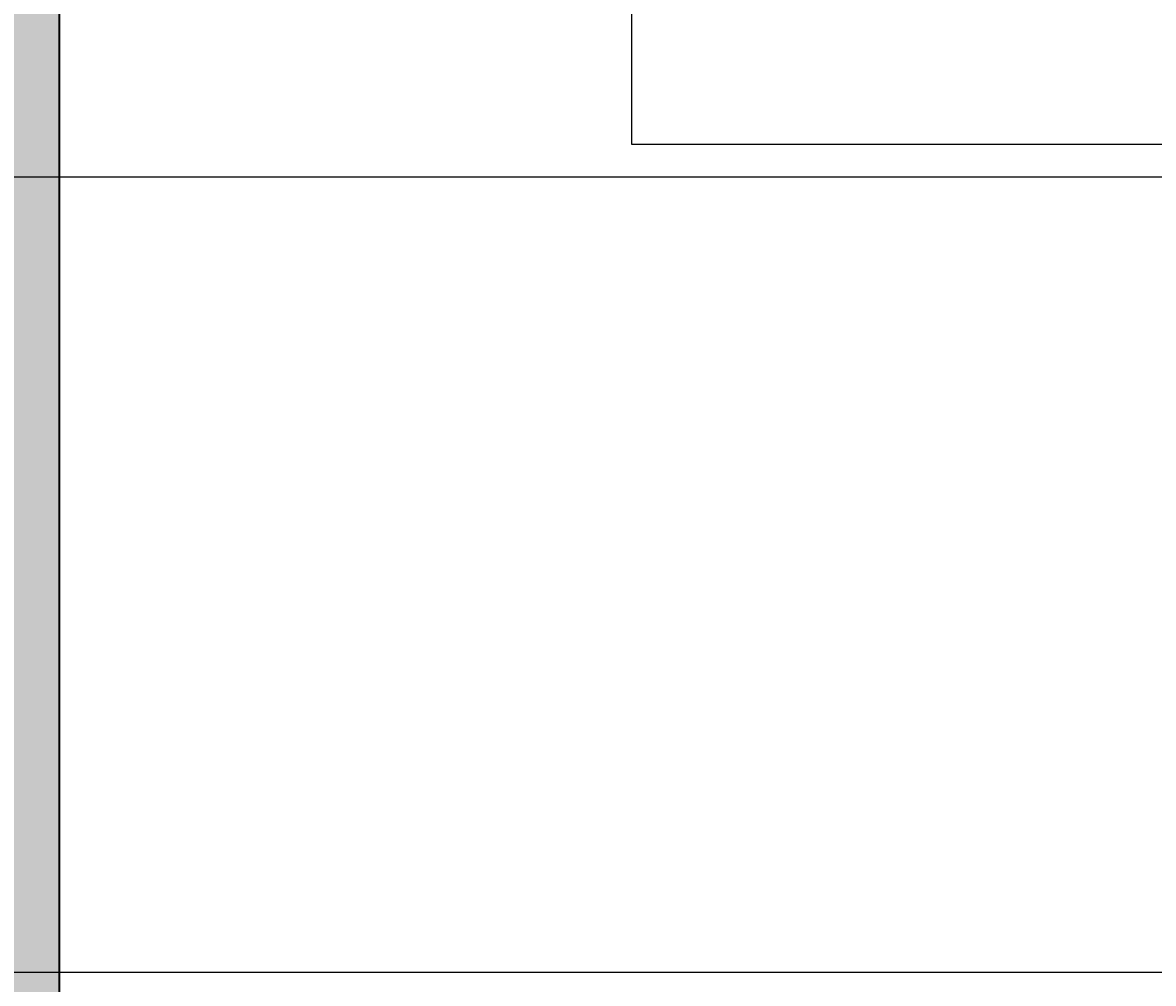
# Model space of a CAD drawing. Units: inches. Extents: x -5 to 330, y -522 to 40.
# Tile 5 of 23: x 32 to 62, y -417 to -391. Entities that reach past the tile are written whole.
import ezdxf

# ---------------------------------------------------------------- set-up
doc = ezdxf.new("R2010")
doc.units = ezdxf.units.IN
doc.header["$MEASUREMENT"] = 0
for name, color, linetype, lineweight in [('A-ANNO-DIMS', 2, 'Continuous', 18), ('A-FLOR-CASE', 8, 'Continuous', 25), ('A-WALL', 7, 'Continuous', 35)]:
    doc.layers.add(name, color=color, linetype=linetype, lineweight=lineweight)
doc.layers.add('A-WALL-PATT', color=18, linetype='Continuous', lineweight=13, true_color=0x000000)
doc.styles.get("Standard").update_dxf_attribs({"font": 'arial.ttf'})
doc.dimstyles.get("Standard").update_dxf_attribs({"dimtxt": 0.18, "dimasz": 0.18, "dimexe": 0.18, "dimexo": 0.0625, "dimgap": 0.09, "dimtad": 0, "dimtih": 1, "dimtoh": 1, "dimdec": 0, "dimzin": 0, "dimdsep": 46, "dimlunit": 3, "dimtxsty": 'Standard', "dimcen": 0.09, "dimadec": 0, "dimazin": 0, "dimtfac": 1, "dimtdec": 0, "dimtofl": 0, "dimtmove": 0, "dimatfit": 3, "dimfxl": 1, "dimtolj": 1, "dimtzin": 0, "dimarcsym": 0})

# ---------------------------------------------------------------- blocks, each defined once
blk = doc.blocks.new('*D40')
at = {"layer": 'A-ANNO-DIMS', "color": 0, "lineweight": -2, "transparency": 16777216}
for p, q in [((32.51, -246.706), (32.51, -522.309)), ((79.01, -246.706), (79.01, -522.309)), ((32.69, -522.129), (55.151, -522.129)), ((78.83, -522.129), (56.369, -522.129))]:
    blk.add_line(p, q, dxfattribs=at)
at = {"layer": 'A-ANNO-DIMS', "color": 0, "transparency": 16777216}
for points in [[(32.69, -522.099), (32.69, -522.159), (32.51, -522.129)], [(78.83, -522.099), (78.83, -522.159), (79.01, -522.129)]]:
    blk.add_solid(points, dxfattribs=at)
at = {"layer": 'Defpoints', "color": 0, "transparency": 16777216}
for p in [(32.51, -246.644), (79.01, -246.644), (79.01, -522.129)]:
    blk.add_point(p, dxfattribs=at)
at = {"layer": 'A-ANNO-DIMS', "color": 0, "transparency": 16777216, "insert": (55.76, -522.129), "char_height": 0.18, "attachment_point": 5}
blk.add_mtext('\\A1;3\'-10 1/2"', dxfattribs=at)
blk = doc.blocks.new('*D49')
at = {"layer": 'A-ANNO-DIMS', "color": 0, "lineweight": -2, "transparency": 16777216}
for p, q in [((62.948, -394.834), (-3.655, -394.834)), ((-3.475, -395.014), (-3.475, -405.506)), ((-3.475, -416.364), (-3.475, -405.872)), ((62.948, -416.544), (-3.655, -416.544))]:
    blk.add_line(p, q, dxfattribs=at)
at = {"layer": 'A-ANNO-DIMS', "color": 0, "transparency": 16777216}
for points in [[(-3.505, -395.014), (-3.445, -395.014), (-3.475, -394.834)], [(-3.505, -416.364), (-3.445, -416.364), (-3.475, -416.544)]]:
    blk.add_solid(points, dxfattribs=at)
at = {"layer": 'Defpoints', "color": 0, "transparency": 16777216}
for p in [(63.01, -394.834), (-3.475, -416.544), (63.01, -416.544)]:
    blk.add_point(p, dxfattribs=at)
at = {"layer": 'A-ANNO-DIMS', "color": 0, "transparency": 16777216, "insert": (-3.475, -405.689), "char_height": 0.18, "attachment_point": 5}
blk.add_mtext('\\A1;1\'-9 1/2"', dxfattribs=at)

msp = doc.modelspace()

# ---------------------------------------------------------------- hatches: boundary and pattern name
at = {"layer": 'A-WALL-PATT'}
h = msp.add_hatch(color=256, dxfattribs=at)
h.dxf.hatch_style = 1
h.paths.add_polyline_path([(164.01, -44.152), (159.51, -44.152), (159.51, -153.144), (164.01, -153.144)], flags=17)
h.paths.add_polyline_path([(224.01, -188.144), (272.01, -188.144), (272.01, -218.144), (260.01, -218.144), (260.01, -222.644), (272.01, -222.644), (272.01, -292.644), (159.01, -292.644), (159.01, -297.144), (272.01, -297.144), (272.01, -417.144), (245.51, -417.144), (245.51, -426.144), (272.01, -426.144), (272.01, -495.144), (281.01, -495.144), (281.01, 12.356), (23.51, 12.356), (23.51, -426.144), (62.918, -426.144), (62.918, -417.144), (32.51, -417.144), (32.51, -297.144), (48.129, -297.144), (48.129, -292.644), (32.51, -292.644), (32.51, -140.644), (133.51, -140.644), (133.51, -131.644), (32.51, -131.644), (32.51, 3.356), (159.51, 3.356), (164.01, 3.356), (220.01, 3.356), (224.51, 3.356), (272.01, 3.356), (272.01, -179.144), (159.51, -179.144), (159.51, -188.144), (219.51, -188.144), (219.51, -266.644), (224.01, -266.644), (224.01, -222.644), (236.01, -222.644), (236.01, -218.144), (224.01, -218.144)])
h.paths.add_polyline_path([(133.01, -292.644), (128.51, -292.644), (128.51, -297.144), (128.51, -417.144), (122.918, -417.144), (122.918, -426.144), (133.01, -426.144)], flags=17)
h.paths.add_polyline_path([(185.51, -417.144), (159.01, -417.144), (159.01, -426.144), (185.51, -426.144)], flags=17)
h.paths.add_polyline_path([(133.51, -140.644), (129.01, -140.644), (129.01, -246.644), (133.51, -246.644)], flags=17)
h.paths.add_polyline_path([(246.01, -48.644), (224.51, -48.644), (224.51, -27.627), (220.01, -27.627), (220.01, -48.644), (198.604, -48.644), (198.604, -53.144), (246.01, -53.144)], flags=17)

# ---------------------------------------------------------------- linework, layer by layer
at = {"layer": 'A-FLOR-CASE'}
for p, q in [((48.129, -297.144), (48.129, -393.928)), ((48.129, -393.928), (128.51, -393.928))]:
    msp.add_line(p, q, dxfattribs=at)
at = {"layer": 'A-WALL'}
msp.add_line((32.51, -297.144), (32.51, -417.144), dxfattribs=at)

# ---------------------------------------------------------------- dimensions: what is measured, and where the dimension line sits
at = {"layer": 'A-ANNO-DIMS'}
dim = msp.add_linear_dim(base=(79.01, -522.129), p1=(32.51, -246.644), p2=(79.01, -246.644), dimstyle='Standard', override={"dimdec": 1, "dimlfac": 1, "dimrnd": 0, "dimzin": 1, "dimdsep": 46, "dimlunit": 4, "dimfrac": 2}, dxfattribs=at)
dim.commit()
dim.dimension.update_dxf_attribs({"geometry": '*D40', "text_midpoint": (55.76, -522.129)})
dim = msp.add_linear_dim(base=(-3.475, -416.544), p1=(63.01, -394.834), p2=(63.01, -416.544), angle=90, dimstyle='Standard', override={"dimdec": 1, "dimlfac": 1, "dimrnd": 0, "dimzin": 1, "dimdsep": 46, "dimlunit": 4, "dimfrac": 2}, dxfattribs=at)
dim.commit()
dim.dimension.update_dxf_attribs({"geometry": '*D49', "text_midpoint": (-3.475, -405.689)})

doc.saveas('drawing.dxf')
